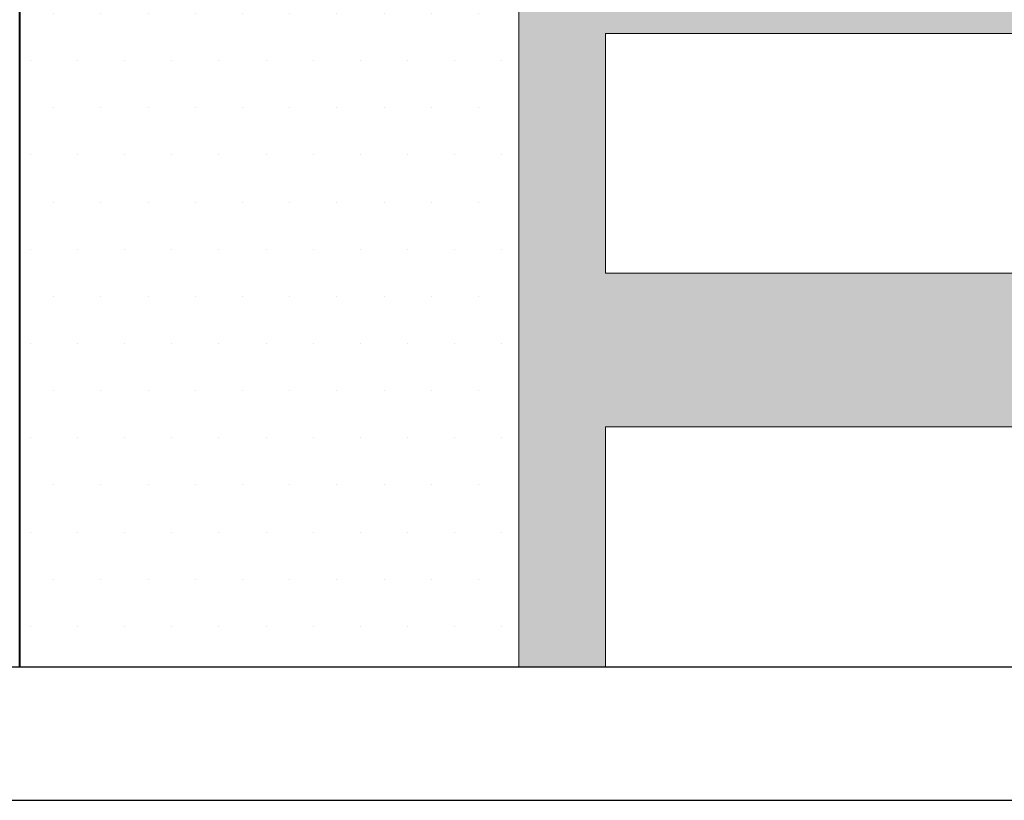
# Model space of a CAD drawing. Units: inches. Extents: x 459864 to 460310, y 324185 to 324787.
# Tile 2 of 112: x 460061 to 460094, y 324195 to 324221. Entities that reach past the tile are written whole.
import ezdxf

# ---------------------------------------------------------------- set-up
doc = ezdxf.new("R2010")
doc.units = ezdxf.units.IN
for name, color, linetype, lineweight in [('A-WALL', 7, 'Continuous', 40), ('C-PROP', 7, 'Continuous', 30), ('L-HRDS', 9, 'Continuous', 18), ('L-SITE-PATT', 252, 'Continuous', 13)]:
    doc.layers.add(name, color=color, linetype=linetype, lineweight=lineweight)

msp = doc.modelspace()

# ---------------------------------------------------------------- hatches: boundary and pattern name
at = {"layer": 'L-SITE-PATT'}
h = msp.add_hatch(dxfattribs=at)
h.set_pattern_fill('DOTS', color=256)
h.paths.add_polyline_path([(460269.804, 324283.483), (460247.115, 324283.483), (460121.929, 324283.483), (460121.929, 324252.473), (460117.429, 324252.473), (460110.124, 324252.473), (460110.124, 324243.287), (460080.83, 324243.287), (460080.83, 324252.473), (460061.115, 324252.473), (460061.115, 324251.882), (460077.909, 324251.882), (460077.909, 324199.483), (460080.83, 324199.483), (460080.83, 324207.553), (460110.124, 324207.553), (460110.124, 324199.483), (460110.813, 324199.483), (460262.115, 324199.483), (460269.804, 324199.483)], flags=17)
edge = h.paths.add_edge_path(flags=0)
edge.add_ellipse((460222.59, 324263.813), major_axis=(-8.485, 8.485), ratio=1, start_angle=405, end_angle=495, ccw=False)
edge.add_line((460214.821, 324254.66), (460214.832, 324254.666))
edge.add_ellipse((460222.59, 324263.813), major_axis=(-8.485, 8.485), ratio=1, start_angle=405, end_angle=495, ccw=False)
edge.add_line((460210.759, 324261.781), (460210.768, 324261.787))
edge.add_ellipse((460222.59, 324263.813), major_axis=(-8.485, 8.485), ratio=1, start_angle=405, end_angle=495, ccw=False)
edge.add_ellipse((460222.59, 324263.813), major_axis=(-8.485, 8.485), ratio=1, start_angle=392.754, end_angle=405, ccw=False)
edge.add_ellipse((460222.59, 324263.813), major_axis=(-8.485, 8.485), ratio=1, start_angle=380.9347, end_angle=392.754, ccw=False)
edge.add_line((460211.337, 324267.985), (460211.34, 324267.985))
edge.add_ellipse((460222.59, 324263.813), major_axis=(-8.485, 8.485), ratio=1, start_angle=380.9347, end_angle=392.754, ccw=False)
edge.add_ellipse((460222.59, 324263.813), major_axis=(-8.485, 8.485), ratio=1, start_angle=347.9015, end_angle=380.9347, ccw=False)
edge.add_ellipse((460222.59, 324263.813), major_axis=(-8.485, 8.485), ratio=1, start_angle=327.0619, end_angle=347.9015, ccw=False)
edge.add_ellipse((460222.59, 324263.813), major_axis=(-8.485, 8.485), ratio=1, start_angle=278.3246, end_angle=327.0619, ccw=False)
edge.add_line((460225.158, 324275.536), (460225.158, 324275.535))
edge.add_ellipse((460222.59, 324263.813), major_axis=(-8.485, 8.485), ratio=1, start_angle=278.3246, end_angle=327.0619, ccw=False)
edge.add_ellipse((460222.59, 324263.813), major_axis=(-8.485, 8.485), ratio=1, start_angle=260.6436, end_angle=278.3246, ccw=False)
edge.add_ellipse((460222.59, 324263.813), major_axis=(-8.485, 8.485), ratio=1, start_angle=225, end_angle=260.6436, ccw=False)
edge.add_line((460234.509, 324265.243), (460234.501, 324265.239))
edge.add_ellipse((460222.59, 324263.813), major_axis=(-8.485, 8.485), ratio=1, start_angle=225, end_angle=260.6436, ccw=False)
edge.add_ellipse((460222.59, 324263.813), major_axis=(-8.485, 8.485), ratio=1, start_angle=495, end_angle=585, ccw=False)
edge.add_line((460234.437, 324261.861), (460234.424, 324261.858))
edge.add_ellipse((460222.59, 324263.813), major_axis=(-8.485, 8.485), ratio=1, start_angle=495, end_angle=585, ccw=False)
edge.add_line((460227.95, 324253.067), (460227.946, 324253.083))
edge.add_ellipse((460222.59, 324263.813), major_axis=(-8.485, 8.485), ratio=1, start_angle=495, end_angle=585, ccw=False)
edge.add_line((460226.223, 324252.369), (460226.211, 324252.38))
edge.add_ellipse((460222.59, 324263.813), major_axis=(-8.485, 8.485), ratio=1, start_angle=495, end_angle=585, ccw=False)
h.paths.add_polyline_path([(460219.651, 324254.347), (460218.461, 324253.545), (460218.275, 324254.789), (460219.642, 324256.542), (460219.625, 324260.848), (460216.11, 324257.333), (460214.35, 324256.978), (460215.416, 324259.356), (460212.524, 324258.496), (460213.137, 324259.93), (460218.507, 324263.813), (460222.59, 324263.813), (460222.59, 324267.807), (460218.176, 324272.212), (460219.026, 324274.639), (460222.59, 324272.811), (460222.59, 324275.423), (460223.057, 324274.825), (460222.675, 324273.492), (460225.912, 324267.135), (460219.625, 324260.848)], flags=0)
edge = h.paths.add_edge_path(flags=0)
edge.add_ellipse((460194.576, 324264.046), major_axis=(-8.485, 8.485), ratio=1, start_angle=495, end_angle=585, ccw=False)
edge.add_line((460199.936, 324253.3), (460199.932, 324253.316))
edge.add_ellipse((460194.576, 324264.046), major_axis=(-8.485, 8.485), ratio=1, start_angle=495, end_angle=585, ccw=False)
edge.add_line((460198.208, 324252.603), (460198.196, 324252.613))
edge.add_ellipse((460194.576, 324264.046), major_axis=(-8.485, 8.485), ratio=1, start_angle=495, end_angle=585, ccw=False)
edge.add_ellipse((460194.576, 324264.046), major_axis=(-8.485, 8.485), ratio=1, start_angle=405, end_angle=495, ccw=False)
edge.add_line((460186.806, 324254.893), (460186.817, 324254.899))
edge.add_ellipse((460194.576, 324264.046), major_axis=(-8.485, 8.485), ratio=1, start_angle=405, end_angle=495, ccw=False)
edge.add_line((460182.744, 324262.014), (460182.753, 324262.02))
edge.add_ellipse((460194.576, 324264.046), major_axis=(-8.485, 8.485), ratio=1, start_angle=405, end_angle=495, ccw=False)
edge.add_ellipse((460194.576, 324264.046), major_axis=(-8.485, 8.485), ratio=1, start_angle=392.754, end_angle=405, ccw=False)
edge.add_ellipse((460194.576, 324264.046), major_axis=(-8.485, 8.485), ratio=1, start_angle=380.9347, end_angle=392.754, ccw=False)
edge.add_line((460183.323, 324268.218), (460183.326, 324268.218))
edge.add_ellipse((460194.576, 324264.046), major_axis=(-8.485, 8.485), ratio=1, start_angle=380.9347, end_angle=392.754, ccw=False)
edge.add_ellipse((460194.576, 324264.046), major_axis=(-8.485, 8.485), ratio=1, start_angle=347.9015, end_angle=380.9347, ccw=False)
edge.add_ellipse((460194.576, 324264.046), major_axis=(-8.485, 8.485), ratio=1, start_angle=327.0619, end_angle=347.9015, ccw=False)
edge.add_ellipse((460194.576, 324264.046), major_axis=(-8.485, 8.485), ratio=1, start_angle=278.3246, end_angle=327.0619, ccw=False)
edge.add_line((460197.144, 324275.769), (460197.143, 324275.768))
edge.add_ellipse((460194.576, 324264.046), major_axis=(-8.485, 8.485), ratio=1, start_angle=278.3246, end_angle=327.0619, ccw=False)
edge.add_ellipse((460194.576, 324264.046), major_axis=(-8.485, 8.485), ratio=1, start_angle=260.6436, end_angle=278.3246, ccw=False)
edge.add_ellipse((460194.576, 324264.046), major_axis=(-8.485, 8.485), ratio=1, start_angle=225, end_angle=260.6436, ccw=False)
edge.add_line((460206.494, 324265.476), (460206.487, 324265.473))
edge.add_ellipse((460194.576, 324264.046), major_axis=(-8.485, 8.485), ratio=1, start_angle=225, end_angle=260.6436, ccw=False)
edge.add_ellipse((460194.576, 324264.046), major_axis=(-8.485, 8.485), ratio=1, start_angle=495, end_angle=585, ccw=False)
edge.add_line((460206.422, 324262.094), (460206.409, 324262.091))
h.paths.add_polyline_path([(460191.61, 324261.081), (460191.637, 324254.58), (460190.447, 324253.778), (460190.261, 324255.023), (460191.628, 324256.775), (460191.61, 324261.081), (460188.096, 324257.566), (460186.335, 324257.211), (460187.402, 324259.589), (460184.509, 324258.729), (460185.123, 324260.163), (460190.493, 324264.046), (460194.576, 324264.046), (460194.576, 324268.04), (460190.161, 324272.446), (460191.011, 324274.872), (460194.576, 324273.044), (460194.576, 324275.657), (460195.043, 324275.058), (460194.661, 324273.725), (460197.897, 324267.368)], flags=0)
edge = h.paths.add_edge_path(flags=0)
edge.add_ellipse((460252.912, 324263.578), major_axis=(-8.485, 8.485), ratio=1, start_angle=405, end_angle=495, ccw=False)
edge.add_line((460241.081, 324261.545), (460241.089, 324261.551))
edge.add_ellipse((460252.912, 324263.578), major_axis=(-8.485, 8.485), ratio=1, start_angle=405, end_angle=495, ccw=False)
edge.add_ellipse((460252.912, 324263.578), major_axis=(-8.485, 8.485), ratio=1, start_angle=392.754, end_angle=405, ccw=False)
edge.add_ellipse((460252.912, 324263.578), major_axis=(-8.485, 8.485), ratio=1, start_angle=380.9347, end_angle=392.754, ccw=False)
edge.add_line((460241.659, 324267.749), (460241.662, 324267.749))
edge.add_ellipse((460252.912, 324263.578), major_axis=(-8.485, 8.485), ratio=1, start_angle=380.9347, end_angle=392.754, ccw=False)
edge.add_ellipse((460252.912, 324263.578), major_axis=(-8.485, 8.485), ratio=1, start_angle=347.9015, end_angle=380.9347, ccw=False)
edge.add_ellipse((460252.912, 324263.578), major_axis=(-8.485, 8.485), ratio=1, start_angle=327.0619, end_angle=347.9015, ccw=False)
edge.add_ellipse((460252.912, 324263.578), major_axis=(-8.485, 8.485), ratio=1, start_angle=278.3246, end_angle=327.0619, ccw=False)
edge.add_line((460255.48, 324275.3), (460255.479, 324275.299))
edge.add_ellipse((460252.912, 324263.578), major_axis=(-8.485, 8.485), ratio=1, start_angle=278.3246, end_angle=327.0619, ccw=False)
edge.add_ellipse((460252.912, 324263.578), major_axis=(-8.485, 8.485), ratio=1, start_angle=260.6436, end_angle=278.3246, ccw=False)
edge.add_ellipse((460252.912, 324263.578), major_axis=(-8.485, 8.485), ratio=1, start_angle=225, end_angle=260.6436, ccw=False)
edge.add_line((460264.83, 324265.007), (460264.823, 324265.004))
edge.add_ellipse((460252.912, 324263.578), major_axis=(-8.485, 8.485), ratio=1, start_angle=225, end_angle=260.6436, ccw=False)
edge.add_ellipse((460252.912, 324263.578), major_axis=(-8.485, 8.485), ratio=1, start_angle=495, end_angle=585, ccw=False)
edge.add_line((460264.758, 324261.626), (460264.745, 324261.622))
edge.add_ellipse((460252.912, 324263.578), major_axis=(-8.485, 8.485), ratio=1, start_angle=495, end_angle=585, ccw=False)
edge.add_line((460258.272, 324252.832), (460258.268, 324252.848))
edge.add_ellipse((460252.912, 324263.578), major_axis=(-8.485, 8.485), ratio=1, start_angle=495, end_angle=585, ccw=False)
edge.add_line((460256.545, 324252.134), (460256.533, 324252.144))
edge.add_ellipse((460252.912, 324263.578), major_axis=(-8.485, 8.485), ratio=1, start_angle=495, end_angle=585, ccw=False)
edge.add_ellipse((460252.912, 324263.578), major_axis=(-8.485, 8.485), ratio=1, start_angle=405, end_angle=495, ccw=False)
edge.add_line((460245.143, 324254.424), (460245.153, 324254.43))
h.paths.add_polyline_path([(460244.672, 324256.742), (460245.738, 324259.12), (460242.846, 324258.26), (460243.459, 324259.694), (460248.829, 324263.578), (460252.912, 324263.578), (460252.912, 324267.571), (460248.497, 324271.977), (460249.348, 324274.403), (460252.912, 324272.576), (460252.912, 324275.188), (460253.379, 324274.589), (460252.997, 324273.257), (460256.233, 324266.899), (460249.946, 324260.612), (460249.973, 324254.111), (460248.783, 324253.309), (460248.597, 324254.554), (460249.964, 324256.306), (460249.946, 324260.612), (460246.432, 324257.097)], flags=0)
edge = h.paths.add_edge_path(flags=0)
edge.add_ellipse((460167.439, 324262.833), major_axis=(-8.485, 8.485), ratio=1, start_angle=495, end_angle=585, ccw=False)
edge.add_line((460172.799, 324252.087), (460172.795, 324252.103))
edge.add_ellipse((460167.439, 324262.833), major_axis=(-8.485, 8.485), ratio=1, start_angle=495, end_angle=585, ccw=False)
edge.add_line((460171.071, 324251.389), (460171.059, 324251.399))
edge.add_ellipse((460167.439, 324262.833), major_axis=(-8.485, 8.485), ratio=1, start_angle=495, end_angle=585, ccw=False)
edge.add_ellipse((460167.439, 324262.833), major_axis=(-8.485, 8.485), ratio=1, start_angle=405, end_angle=495, ccw=False)
edge.add_line((460159.669, 324253.679), (460159.68, 324253.685))
edge.add_ellipse((460167.439, 324262.833), major_axis=(-8.485, 8.485), ratio=1, start_angle=405, end_angle=495, ccw=False)
edge.add_line((460155.607, 324260.8), (460155.616, 324260.806))
edge.add_ellipse((460167.439, 324262.833), major_axis=(-8.485, 8.485), ratio=1, start_angle=405, end_angle=495, ccw=False)
edge.add_ellipse((460167.439, 324262.833), major_axis=(-8.485, 8.485), ratio=1, start_angle=392.754, end_angle=405, ccw=False)
edge.add_ellipse((460167.439, 324262.833), major_axis=(-8.485, 8.485), ratio=1, start_angle=380.9347, end_angle=392.754, ccw=False)
edge.add_line((460156.185, 324267.005), (460156.189, 324267.005))
edge.add_ellipse((460167.439, 324262.833), major_axis=(-8.485, 8.485), ratio=1, start_angle=380.9347, end_angle=392.754, ccw=False)
edge.add_ellipse((460167.439, 324262.833), major_axis=(-8.485, 8.485), ratio=1, start_angle=347.9015, end_angle=380.9347, ccw=False)
edge.add_ellipse((460167.439, 324262.833), major_axis=(-8.485, 8.485), ratio=1, start_angle=327.0619, end_angle=347.9015, ccw=False)
edge.add_ellipse((460167.439, 324262.833), major_axis=(-8.485, 8.485), ratio=1, start_angle=278.3246, end_angle=327.0619, ccw=False)
edge.add_line((460170.007, 324274.556), (460170.006, 324274.554))
edge.add_ellipse((460167.439, 324262.833), major_axis=(-8.485, 8.485), ratio=1, start_angle=278.3246, end_angle=327.0619, ccw=False)
edge.add_ellipse((460167.439, 324262.833), major_axis=(-8.485, 8.485), ratio=1, start_angle=260.6436, end_angle=278.3246, ccw=False)
edge.add_ellipse((460167.439, 324262.833), major_axis=(-8.485, 8.485), ratio=1, start_angle=225, end_angle=260.6436, ccw=False)
edge.add_line((460179.357, 324264.262), (460179.35, 324264.259))
edge.add_ellipse((460167.439, 324262.833), major_axis=(-8.485, 8.485), ratio=1, start_angle=225, end_angle=260.6436, ccw=False)
edge.add_ellipse((460167.439, 324262.833), major_axis=(-8.485, 8.485), ratio=1, start_angle=495, end_angle=585, ccw=False)
edge.add_line((460179.285, 324260.881), (460179.272, 324260.877))
h.paths.add_polyline_path([(460164.473, 324259.867), (460164.5, 324253.366), (460163.31, 324252.565), (460163.124, 324253.809), (460164.491, 324255.561), (460164.473, 324259.867), (460160.958, 324256.353), (460159.198, 324255.998), (460160.265, 324258.375), (460157.372, 324257.515), (460157.986, 324258.949), (460163.356, 324262.833), (460167.439, 324262.833), (460167.439, 324266.826), (460163.024, 324271.232), (460163.874, 324273.659), (460167.439, 324271.831), (460167.439, 324274.443), (460167.905, 324273.844), (460167.524, 324272.512), (460170.76, 324266.154)], flags=0)
edge = h.paths.add_edge_path(flags=0)
edge.add_ellipse((460140.758, 324262.37), major_axis=(-8.485, 8.485), ratio=1, start_angle=495, end_angle=585, ccw=False)
edge.add_line((460146.118, 324251.624), (460146.114, 324251.639))
edge.add_ellipse((460140.758, 324262.37), major_axis=(-8.485, 8.485), ratio=1, start_angle=495, end_angle=585, ccw=False)
edge.add_line((460144.391, 324250.926), (460144.379, 324250.936))
edge.add_ellipse((460140.758, 324262.37), major_axis=(-8.485, 8.485), ratio=1, start_angle=495, end_angle=585, ccw=False)
edge.add_ellipse((460140.758, 324262.37), major_axis=(-8.485, 8.485), ratio=1, start_angle=405, end_angle=495, ccw=False)
edge.add_line((460132.989, 324253.216), (460132.999, 324253.222))
edge.add_ellipse((460140.758, 324262.37), major_axis=(-8.485, 8.485), ratio=1, start_angle=405, end_angle=495, ccw=False)
edge.add_line((460128.927, 324260.337), (460128.935, 324260.343))
edge.add_ellipse((460140.758, 324262.37), major_axis=(-8.485, 8.485), ratio=1, start_angle=405, end_angle=495, ccw=False)
edge.add_ellipse((460140.758, 324262.37), major_axis=(-8.485, 8.485), ratio=1, start_angle=392.754, end_angle=405, ccw=False)
edge.add_ellipse((460140.758, 324262.37), major_axis=(-8.485, 8.485), ratio=1, start_angle=380.9347, end_angle=392.754, ccw=False)
edge.add_line((460129.505, 324266.541), (460129.508, 324266.541))
edge.add_ellipse((460140.758, 324262.37), major_axis=(-8.485, 8.485), ratio=1, start_angle=380.9347, end_angle=392.754, ccw=False)
edge.add_ellipse((460140.758, 324262.37), major_axis=(-8.485, 8.485), ratio=1, start_angle=347.9015, end_angle=380.9347, ccw=False)
edge.add_ellipse((460140.758, 324262.37), major_axis=(-8.485, 8.485), ratio=1, start_angle=327.0619, end_angle=347.9015, ccw=False)
edge.add_ellipse((460140.758, 324262.37), major_axis=(-8.485, 8.485), ratio=1, start_angle=278.3246, end_angle=327.0619, ccw=False)
edge.add_line((460143.326, 324274.092), (460143.325, 324274.091))
edge.add_ellipse((460140.758, 324262.37), major_axis=(-8.485, 8.485), ratio=1, start_angle=278.3246, end_angle=327.0619, ccw=False)
edge.add_ellipse((460140.758, 324262.37), major_axis=(-8.485, 8.485), ratio=1, start_angle=260.6436, end_angle=278.3246, ccw=False)
edge.add_ellipse((460140.758, 324262.37), major_axis=(-8.485, 8.485), ratio=1, start_angle=225, end_angle=260.6436, ccw=False)
edge.add_line((460152.677, 324263.799), (460152.669, 324263.796))
edge.add_ellipse((460140.758, 324262.37), major_axis=(-8.485, 8.485), ratio=1, start_angle=225, end_angle=260.6436, ccw=False)
edge.add_ellipse((460140.758, 324262.37), major_axis=(-8.485, 8.485), ratio=1, start_angle=495, end_angle=585, ccw=False)
edge.add_line((460152.604, 324260.418), (460152.592, 324260.414))
h.paths.add_polyline_path([(460137.792, 324259.404), (460137.819, 324252.903), (460136.629, 324252.101), (460136.443, 324253.346), (460137.81, 324255.098), (460137.792, 324259.404), (460134.278, 324255.889), (460132.518, 324255.534), (460133.584, 324257.912), (460130.692, 324257.052), (460131.305, 324258.486), (460136.675, 324262.37), (460140.758, 324262.37), (460140.758, 324266.363), (460136.343, 324270.769), (460137.194, 324273.195), (460140.758, 324271.367), (460140.758, 324273.98), (460141.225, 324273.381), (460140.843, 324272.049), (460144.079, 324265.691)], flags=0)
h.paths.add_polyline_path([(460110.124, 324227.414), (460080.83, 324227.414), (460080.83, 324235.484), (460110.124, 324235.484)], flags=16)
h.paths.add_polyline_path([(460110.124, 324220.797), (460110.124, 324212.727), (460080.83, 324212.727), (460080.83, 324220.797)], flags=16)
h.paths.add_polyline_path([(460269.804, 324283.483), (460247.115, 324283.483), (460121.929, 324283.483), (460121.929, 324252.473), (460117.429, 324252.473), (460110.124, 324252.473), (460110.124, 324243.287), (460080.83, 324243.287), (460080.83, 324252.473), (460061.115, 324252.473), (460061.115, 324251.882), (460077.909, 324251.882), (460077.909, 324199.483), (460080.83, 324199.483), (460080.83, 324207.553), (460110.124, 324207.553), (460110.124, 324199.483), (460262.115, 324199.483), (460269.804, 324199.483)], flags=17)
h.paths.add_polyline_path([(460219.651, 324254.347), (460218.461, 324253.545), (460218.275, 324254.789), (460219.642, 324256.542), (460219.625, 324260.848), (460216.11, 324257.333), (460214.35, 324256.978), (460215.416, 324259.356), (460212.524, 324258.496), (460213.137, 324259.93), (460218.507, 324263.813), (460222.59, 324263.813), (460220.18, 324266.223), (460215.461, 324265.308), (460211.835, 324266.137), (460216.247, 324267.985), (460218.418, 324267.985), (460222.59, 324263.813), (460222.59, 324267.807), (460218.176, 324272.212), (460219.026, 324274.639), (460222.59, 324272.811), (460222.59, 324275.423), (460223.057, 324274.825), (460222.675, 324273.492), (460225.912, 324267.135), (460222.59, 324263.813), (460231.383, 324263.813), (460228.485, 324262.488), (460224.425, 324261.978), (460228.68, 324257.724), (460228.966, 324254.791), (460227.142, 324256.537), (460227.542, 324254.819), (460227.333, 324253.614), (460222.59, 324259.985), (460222.59, 324255.497), (460221.377, 324256.541), (460220.576, 324261.799), (460219.625, 324260.848)], flags=0)
h.paths.add_polyline_path([(460199.127, 324256.77), (460199.528, 324255.052), (460199.319, 324253.848), (460194.576, 324260.218), (460194.576, 324255.73), (460193.363, 324256.774), (460192.561, 324262.032), (460191.61, 324261.081), (460191.637, 324254.58), (460190.447, 324253.778), (460190.261, 324255.023), (460191.628, 324256.775), (460191.61, 324261.081), (460188.096, 324257.566), (460186.335, 324257.211), (460187.402, 324259.589), (460184.509, 324258.729), (460185.123, 324260.163), (460190.493, 324264.046), (460194.576, 324264.046), (460192.166, 324266.456), (460187.446, 324265.541), (460183.82, 324266.37), (460188.232, 324268.218), (460190.404, 324268.218), (460194.576, 324264.046), (460194.576, 324268.04), (460190.161, 324272.446), (460191.011, 324274.872), (460194.576, 324273.044), (460194.576, 324275.657), (460195.043, 324275.058), (460194.661, 324273.725), (460197.897, 324267.368), (460194.576, 324264.046), (460203.368, 324264.046), (460200.47, 324262.721), (460196.411, 324262.212), (460200.665, 324257.957), (460200.951, 324255.024)], flags=0)
h.paths.add_polyline_path([(460244.672, 324256.742), (460245.738, 324259.12), (460242.846, 324258.26), (460243.459, 324259.694), (460248.829, 324263.578), (460252.912, 324263.578), (460250.502, 324265.987), (460245.783, 324265.072), (460242.156, 324265.901), (460246.568, 324267.749), (460248.74, 324267.749), (460252.912, 324263.578), (460252.912, 324267.571), (460248.497, 324271.977), (460249.348, 324274.403), (460252.912, 324272.576), (460252.912, 324275.188), (460253.379, 324274.589), (460252.997, 324273.257), (460256.233, 324266.899), (460252.912, 324263.578), (460261.705, 324263.578), (460258.806, 324262.252), (460254.747, 324261.743), (460259.002, 324257.488), (460259.288, 324254.555), (460257.463, 324256.301), (460257.864, 324254.583), (460257.655, 324253.379), (460252.912, 324259.749), (460252.912, 324255.261), (460251.699, 324256.305), (460250.897, 324261.563), (460249.946, 324260.612), (460249.973, 324254.111), (460248.783, 324253.309), (460248.597, 324254.554), (460249.964, 324256.306), (460249.946, 324260.612), (460246.432, 324257.097)], flags=0)
h.paths.add_polyline_path([(460173.528, 324256.743), (460173.814, 324253.811), (460171.99, 324255.556), (460172.39, 324253.838), (460172.182, 324252.634), (460167.439, 324259.004), (460167.439, 324254.516), (460166.226, 324255.56), (460165.424, 324260.818), (460164.473, 324259.867), (460164.5, 324253.366), (460163.31, 324252.565), (460163.124, 324253.809), (460164.491, 324255.561), (460164.473, 324259.867), (460160.958, 324256.353), (460159.198, 324255.998), (460160.265, 324258.375), (460157.372, 324257.515), (460157.986, 324258.949), (460163.356, 324262.833), (460167.439, 324262.833), (460165.029, 324265.243), (460160.309, 324264.327), (460156.683, 324265.156), (460161.095, 324267.005), (460163.267, 324267.005), (460167.439, 324262.833), (460167.439, 324266.826), (460163.024, 324271.232), (460163.874, 324273.659), (460167.439, 324271.831), (460167.439, 324274.443), (460167.905, 324273.844), (460167.524, 324272.512), (460170.76, 324266.154), (460167.439, 324262.833), (460176.231, 324262.833), (460173.333, 324261.507), (460169.274, 324260.998)], flags=0)
h.paths.add_polyline_path([(460146.848, 324256.28), (460147.134, 324253.347), (460145.31, 324255.093), (460145.71, 324253.375), (460145.501, 324252.171), (460140.758, 324258.541), (460140.758, 324254.053), (460139.545, 324255.097), (460138.744, 324260.355), (460137.792, 324259.404), (460137.819, 324252.903), (460136.629, 324252.101), (460136.443, 324253.346), (460137.81, 324255.098), (460137.792, 324259.404), (460134.278, 324255.889), (460132.518, 324255.534), (460133.584, 324257.912), (460130.692, 324257.052), (460131.305, 324258.486), (460136.675, 324262.37), (460140.758, 324262.37), (460138.348, 324264.779), (460133.629, 324263.864), (460130.002, 324264.693), (460134.414, 324266.541), (460136.586, 324266.541), (460140.758, 324262.37), (460140.758, 324266.363), (460136.343, 324270.769), (460137.194, 324273.195), (460140.758, 324271.367), (460140.758, 324273.98), (460141.225, 324273.381), (460140.843, 324272.049), (460144.079, 324265.691), (460140.758, 324262.37), (460149.551, 324262.37), (460146.653, 324261.044), (460142.593, 324260.535)], flags=0)
edge = h.paths.add_edge_path()
edge.add_line((460269.804, 324272.549), (460260.881, 324272.549))
edge.add_ellipse((460252.912, 324263.578), major_axis=(-8.485, 8.485), ratio=1, start_angle=260.6436, end_angle=273.3846, ccw=False)
edge.add_line((460262.283, 324271.092), (460262.261, 324271.091))
edge.add_ellipse((460252.912, 324263.578), major_axis=(-8.485, 8.485), ratio=1, start_angle=260.6436, end_angle=273.3846, ccw=False)
edge.add_ellipse((460252.912, 324263.578), major_axis=(-8.485, 8.485), ratio=1, start_angle=225, end_angle=260.6436, ccw=False)
edge.add_line((460263.609, 324269.063), (460263.572, 324269.058))
edge.add_ellipse((460252.912, 324263.578), major_axis=(-8.485, 8.485), ratio=1, start_angle=225, end_angle=260.6436, ccw=False)
edge.add_line((460264.615, 324266.306), (460264.585, 324266.305))
edge.add_ellipse((460252.912, 324263.578), major_axis=(-8.485, 8.485), ratio=1, start_angle=225, end_angle=260.6436, ccw=False)
edge.add_line((460264.83, 324265.007), (460264.823, 324265.004))
edge.add_ellipse((460252.912, 324263.578), major_axis=(-8.485, 8.485), ratio=1, start_angle=225, end_angle=260.6436, ccw=False)
edge.add_ellipse((460252.912, 324263.578), major_axis=(-8.485, 8.485), ratio=1, start_angle=495, end_angle=585, ccw=False)
edge.add_line((460264.758, 324261.626), (460264.745, 324261.622))
edge.add_ellipse((460252.912, 324263.578), major_axis=(-8.485, 8.485), ratio=1, start_angle=495, end_angle=585, ccw=False)
edge.add_line((460263.442, 324257.739), (460263.389, 324257.779))
edge.add_ellipse((460252.912, 324263.578), major_axis=(-8.485, 8.485), ratio=1, start_angle=495, end_angle=585, ccw=False)
edge.add_line((460258.128, 324252.744), (460258.102, 324252.779))
edge.add_ellipse((460252.912, 324263.578), major_axis=(-8.485, 8.485), ratio=1, start_angle=495, end_angle=585, ccw=False)
edge.add_line((460256.545, 324252.134), (460256.533, 324252.144))
edge.add_ellipse((460252.912, 324263.578), major_axis=(-8.485, 8.485), ratio=1, start_angle=495, end_angle=585, ccw=False)
edge.add_ellipse((460252.912, 324263.578), major_axis=(-8.485, 8.485), ratio=1, start_angle=405, end_angle=495, ccw=False)
edge.add_line((460250.594, 324251.78), (460250.605, 324251.82))
edge.add_ellipse((460252.912, 324263.578), major_axis=(-8.485, 8.485), ratio=1, start_angle=405, end_angle=495, ccw=False)
edge.add_line((460245.143, 324254.424), (460245.153, 324254.43))
edge.add_ellipse((460252.912, 324263.578), major_axis=(-8.485, 8.485), ratio=1, start_angle=405, end_angle=495, ccw=False)
edge.add_line((460243.525, 324256.059), (460243.56, 324256.091))
edge.add_ellipse((460252.912, 324263.578), major_axis=(-8.485, 8.485), ratio=1, start_angle=405, end_angle=495, ccw=False)
edge.add_line((460241.44, 324259.893), (460241.522, 324259.896))
edge.add_ellipse((460252.912, 324263.578), major_axis=(-8.485, 8.485), ratio=1, start_angle=405, end_angle=495, ccw=False)
edge.add_line((460241.081, 324261.545), (460241.089, 324261.551))
edge.add_ellipse((460252.912, 324263.578), major_axis=(-8.485, 8.485), ratio=1, start_angle=405, end_angle=495, ccw=False)
edge.add_ellipse((460252.912, 324263.578), major_axis=(-8.485, 8.485), ratio=1, start_angle=392.754, end_angle=405, ccw=False)
edge.add_line((460241.05, 324265.438), (460241.063, 324265.443))
edge.add_ellipse((460252.912, 324263.578), major_axis=(-8.485, 8.485), ratio=1, start_angle=392.754, end_angle=405, ccw=False)
edge.add_ellipse((460252.912, 324263.578), major_axis=(-8.485, 8.485), ratio=1, start_angle=380.9347, end_angle=392.754, ccw=False)
edge.add_line((460241.452, 324267.176), (460241.469, 324267.171))
edge.add_ellipse((460252.912, 324263.578), major_axis=(-8.485, 8.485), ratio=1, start_angle=380.9347, end_angle=392.754, ccw=False)
edge.add_line((460241.659, 324267.749), (460241.662, 324267.749))
edge.add_ellipse((460252.912, 324263.578), major_axis=(-8.485, 8.485), ratio=1, start_angle=380.9347, end_angle=392.754, ccw=False)
edge.add_ellipse((460252.912, 324263.578), major_axis=(-8.485, 8.485), ratio=1, start_angle=356.6154, end_angle=380.9347, ccw=False)
edge.add_line((460244.88, 324272.488), (460244.713, 324272.549))
edge.add_line((460244.713, 324272.549), (460230.817, 324272.549))
edge.add_ellipse((460222.59, 324263.813), major_axis=(-8.485, 8.485), ratio=1, start_angle=260.6436, end_angle=271.7178, ccw=False)
edge.add_ellipse((460222.59, 324263.813), major_axis=(-8.485, 8.485), ratio=1, start_angle=225, end_angle=260.6436, ccw=False)
edge.add_line((460233.287, 324269.299), (460233.25, 324269.294))
edge.add_ellipse((460222.59, 324263.813), major_axis=(-8.485, 8.485), ratio=1, start_angle=225, end_angle=260.6436, ccw=False)
edge.add_line((460234.294, 324266.541), (460234.264, 324266.541))
edge.add_ellipse((460222.59, 324263.813), major_axis=(-8.485, 8.485), ratio=1, start_angle=225, end_angle=260.6436, ccw=False)
edge.add_line((460234.509, 324265.243), (460234.501, 324265.239))
edge.add_ellipse((460222.59, 324263.813), major_axis=(-8.485, 8.485), ratio=1, start_angle=225, end_angle=260.6436, ccw=False)
edge.add_ellipse((460222.59, 324263.813), major_axis=(-8.485, 8.485), ratio=1, start_angle=495, end_angle=585, ccw=False)
edge.add_line((460234.437, 324261.861), (460234.424, 324261.858))
edge.add_ellipse((460222.59, 324263.813), major_axis=(-8.485, 8.485), ratio=1, start_angle=495, end_angle=585, ccw=False)
edge.add_line((460233.121, 324257.975), (460233.068, 324258.015))
edge.add_ellipse((460222.59, 324263.813), major_axis=(-8.485, 8.485), ratio=1, start_angle=495, end_angle=585, ccw=False)
edge.add_line((460227.806, 324252.979), (460227.78, 324253.014))
edge.add_ellipse((460222.59, 324263.813), major_axis=(-8.485, 8.485), ratio=1, start_angle=495, end_angle=585, ccw=False)
edge.add_line((460226.223, 324252.369), (460226.211, 324252.38))
edge.add_ellipse((460222.59, 324263.813), major_axis=(-8.485, 8.485), ratio=1, start_angle=495, end_angle=585, ccw=False)
edge.add_ellipse((460222.59, 324263.813), major_axis=(-8.485, 8.485), ratio=1, start_angle=405, end_angle=495, ccw=False)
edge.add_line((460220.272, 324252.016), (460220.283, 324252.055))
edge.add_ellipse((460222.59, 324263.813), major_axis=(-8.485, 8.485), ratio=1, start_angle=405, end_angle=495, ccw=False)
edge.add_line((460214.821, 324254.66), (460214.832, 324254.666))
edge.add_ellipse((460222.59, 324263.813), major_axis=(-8.485, 8.485), ratio=1, start_angle=405, end_angle=495, ccw=False)
edge.add_line((460213.203, 324256.295), (460213.239, 324256.327))
edge.add_ellipse((460222.59, 324263.813), major_axis=(-8.485, 8.485), ratio=1, start_angle=405, end_angle=495, ccw=False)
edge.add_line((460211.118, 324260.128), (460211.201, 324260.131))
edge.add_ellipse((460222.59, 324263.813), major_axis=(-8.485, 8.485), ratio=1, start_angle=405, end_angle=495, ccw=False)
edge.add_line((460210.759, 324261.781), (460210.768, 324261.787))
edge.add_ellipse((460222.59, 324263.813), major_axis=(-8.485, 8.485), ratio=1, start_angle=405, end_angle=495, ccw=False)
edge.add_ellipse((460222.59, 324263.813), major_axis=(-8.485, 8.485), ratio=1, start_angle=392.754, end_angle=405, ccw=False)
edge.add_line((460210.729, 324265.673), (460210.741, 324265.678))
edge.add_ellipse((460222.59, 324263.813), major_axis=(-8.485, 8.485), ratio=1, start_angle=392.754, end_angle=405, ccw=False)
edge.add_ellipse((460222.59, 324263.813), major_axis=(-8.485, 8.485), ratio=1, start_angle=380.9347, end_angle=392.754, ccw=False)
edge.add_line((460211.13, 324267.412), (460211.147, 324267.407))
edge.add_ellipse((460222.59, 324263.813), major_axis=(-8.485, 8.485), ratio=1, start_angle=380.9347, end_angle=392.754, ccw=False)
edge.add_line((460211.337, 324267.985), (460211.34, 324267.985))
edge.add_ellipse((460222.59, 324263.813), major_axis=(-8.485, 8.485), ratio=1, start_angle=380.9347, end_angle=392.754, ccw=False)
edge.add_ellipse((460222.59, 324263.813), major_axis=(-8.485, 8.485), ratio=1, start_angle=358.2822, end_angle=380.9347, ccw=False)
edge.add_line((460213.705, 324271.902), (460213.709, 324271.869))
edge.add_ellipse((460222.59, 324263.813), major_axis=(-8.485, 8.485), ratio=1, start_angle=358.2822, end_angle=380.9347, ccw=False)
edge.add_line((460214.363, 324272.549), (460203.078, 324272.549))
edge.add_line((460203.078, 324272.549), (460203.06, 324272.531))
edge.add_ellipse((460194.576, 324264.046), major_axis=(-8.485, 8.485), ratio=1, start_angle=260.6436, end_angle=270.1168, ccw=False)
edge.add_line((460203.957, 324271.561), (460203.921, 324271.56))
edge.add_ellipse((460194.576, 324264.046), major_axis=(-8.485, 8.485), ratio=1, start_angle=260.6436, end_angle=270.1168, ccw=False)
edge.add_ellipse((460194.576, 324264.046), major_axis=(-8.485, 8.485), ratio=1, start_angle=225, end_angle=260.6436, ccw=False)
edge.add_line((460205.272, 324269.532), (460205.235, 324269.527))
edge.add_ellipse((460194.576, 324264.046), major_axis=(-8.485, 8.485), ratio=1, start_angle=225, end_angle=260.6436, ccw=False)
edge.add_line((460206.279, 324266.774), (460206.249, 324266.774))
edge.add_ellipse((460194.576, 324264.046), major_axis=(-8.485, 8.485), ratio=1, start_angle=225, end_angle=260.6436, ccw=False)
edge.add_line((460206.494, 324265.476), (460206.487, 324265.473))
edge.add_ellipse((460194.576, 324264.046), major_axis=(-8.485, 8.485), ratio=1, start_angle=225, end_angle=260.6436, ccw=False)
edge.add_ellipse((460194.576, 324264.046), major_axis=(-8.485, 8.485), ratio=1, start_angle=495, end_angle=585, ccw=False)
edge.add_line((460206.422, 324262.094), (460206.409, 324262.091))
edge.add_ellipse((460194.576, 324264.046), major_axis=(-8.485, 8.485), ratio=1, start_angle=495, end_angle=585, ccw=False)
edge.add_line((460205.106, 324258.208), (460205.053, 324258.248))
edge.add_ellipse((460194.576, 324264.046), major_axis=(-8.485, 8.485), ratio=1, start_angle=495, end_angle=585, ccw=False)
edge.add_line((460199.792, 324253.212), (460199.766, 324253.248))
edge.add_ellipse((460194.576, 324264.046), major_axis=(-8.485, 8.485), ratio=1, start_angle=495, end_angle=585, ccw=False)
edge.add_line((460198.208, 324252.603), (460198.196, 324252.613))
edge.add_ellipse((460194.576, 324264.046), major_axis=(-8.485, 8.485), ratio=1, start_angle=495, end_angle=585, ccw=False)
edge.add_ellipse((460194.576, 324264.046), major_axis=(-8.485, 8.485), ratio=1, start_angle=405, end_angle=495, ccw=False)
edge.add_line((460192.258, 324252.249), (460192.268, 324252.289))
edge.add_ellipse((460194.576, 324264.046), major_axis=(-8.485, 8.485), ratio=1, start_angle=405, end_angle=495, ccw=False)
edge.add_line((460186.806, 324254.893), (460186.817, 324254.899))
edge.add_ellipse((460194.576, 324264.046), major_axis=(-8.485, 8.485), ratio=1, start_angle=405, end_angle=495, ccw=False)
edge.add_line((460185.188, 324256.528), (460185.224, 324256.56))
edge.add_ellipse((460194.576, 324264.046), major_axis=(-8.485, 8.485), ratio=1, start_angle=405, end_angle=495, ccw=False)
edge.add_line((460183.104, 324260.362), (460183.186, 324260.365))
edge.add_ellipse((460194.576, 324264.046), major_axis=(-8.485, 8.485), ratio=1, start_angle=405, end_angle=495, ccw=False)
edge.add_line((460182.744, 324262.014), (460182.753, 324262.02))
edge.add_ellipse((460194.576, 324264.046), major_axis=(-8.485, 8.485), ratio=1, start_angle=405, end_angle=495, ccw=False)
edge.add_ellipse((460194.576, 324264.046), major_axis=(-8.485, 8.485), ratio=1, start_angle=392.754, end_angle=405, ccw=False)
edge.add_line((460182.714, 324265.906), (460182.726, 324265.912))
edge.add_ellipse((460194.576, 324264.046), major_axis=(-8.485, 8.485), ratio=1, start_angle=392.754, end_angle=405, ccw=False)
edge.add_ellipse((460194.576, 324264.046), major_axis=(-8.485, 8.485), ratio=1, start_angle=380.9347, end_angle=392.754, ccw=False)
edge.add_line((460183.116, 324267.645), (460183.133, 324267.64))
edge.add_ellipse((460194.576, 324264.046), major_axis=(-8.485, 8.485), ratio=1, start_angle=380.9347, end_angle=392.754, ccw=False)
edge.add_line((460183.323, 324268.218), (460183.326, 324268.218))
edge.add_ellipse((460194.576, 324264.046), major_axis=(-8.485, 8.485), ratio=1, start_angle=380.9347, end_angle=392.754, ccw=False)
edge.add_ellipse((460194.576, 324264.046), major_axis=(-8.485, 8.485), ratio=1, start_angle=359.8832, end_angle=380.9347, ccw=False)
edge.add_line((460184.491, 324270.611), (460184.553, 324270.611))
edge.add_ellipse((460194.576, 324264.046), major_axis=(-8.485, 8.485), ratio=1, start_angle=359.8832, end_angle=380.9347, ccw=False)
edge.add_line((460185.346, 324271.76), (460185.379, 324271.728))
edge.add_ellipse((460194.576, 324264.046), major_axis=(-8.485, 8.485), ratio=1, start_angle=359.8832, end_angle=380.9347, ccw=False)
edge.add_line((460185.697, 324272.086), (460185.633, 324272.549))
edge.add_line((460185.633, 324272.549), (460174.683, 324272.549))
edge.add_line((460174.683, 324272.549), (460174.606, 324272.457))
edge.add_ellipse((460167.439, 324262.833), major_axis=(-8.485, 8.485), ratio=1, start_angle=260.6436, end_angle=278.3246, ccw=False)
edge.add_ellipse((460167.439, 324262.833), major_axis=(-8.485, 8.485), ratio=1, start_angle=225, end_angle=260.6436, ccw=False)
edge.add_line((460178.135, 324268.318), (460178.098, 324268.313))
edge.add_ellipse((460167.439, 324262.833), major_axis=(-8.485, 8.485), ratio=1, start_angle=225, end_angle=260.6436, ccw=False)
edge.add_line((460179.142, 324265.561), (460179.112, 324265.56))
edge.add_ellipse((460167.439, 324262.833), major_axis=(-8.485, 8.485), ratio=1, start_angle=225, end_angle=260.6436, ccw=False)
edge.add_line((460179.357, 324264.262), (460179.35, 324264.259))
edge.add_ellipse((460167.439, 324262.833), major_axis=(-8.485, 8.485), ratio=1, start_angle=225, end_angle=260.6436, ccw=False)
edge.add_ellipse((460167.439, 324262.833), major_axis=(-8.485, 8.485), ratio=1, start_angle=495, end_angle=585, ccw=False)
edge.add_line((460179.285, 324260.881), (460179.272, 324260.877))
edge.add_ellipse((460167.439, 324262.833), major_axis=(-8.485, 8.485), ratio=1, start_angle=495, end_angle=585, ccw=False)
edge.add_line((460177.969, 324256.994), (460177.916, 324257.034))
edge.add_ellipse((460167.439, 324262.833), major_axis=(-8.485, 8.485), ratio=1, start_angle=495, end_angle=585, ccw=False)
edge.add_line((460172.655, 324251.999), (460172.629, 324252.034))
edge.add_ellipse((460167.439, 324262.833), major_axis=(-8.485, 8.485), ratio=1, start_angle=495, end_angle=585, ccw=False)
edge.add_line((460171.071, 324251.389), (460171.059, 324251.399))
edge.add_ellipse((460167.439, 324262.833), major_axis=(-8.485, 8.485), ratio=1, start_angle=495, end_angle=585, ccw=False)
edge.add_ellipse((460167.439, 324262.833), major_axis=(-8.485, 8.485), ratio=1, start_angle=405, end_angle=495, ccw=False)
edge.add_line((460165.121, 324251.036), (460165.131, 324251.075))
edge.add_ellipse((460167.439, 324262.833), major_axis=(-8.485, 8.485), ratio=1, start_angle=405, end_angle=495, ccw=False)
edge.add_line((460159.669, 324253.679), (460159.68, 324253.685))
edge.add_ellipse((460167.439, 324262.833), major_axis=(-8.485, 8.485), ratio=1, start_angle=405, end_angle=495, ccw=False)
edge.add_line((460158.051, 324255.314), (460158.087, 324255.347))
edge.add_ellipse((460167.439, 324262.833), major_axis=(-8.485, 8.485), ratio=1, start_angle=405, end_angle=495, ccw=False)
edge.add_line((460155.967, 324259.148), (460156.049, 324259.151))
edge.add_ellipse((460167.439, 324262.833), major_axis=(-8.485, 8.485), ratio=1, start_angle=405, end_angle=495, ccw=False)
edge.add_line((460155.607, 324260.8), (460155.616, 324260.806))
edge.add_ellipse((460167.439, 324262.833), major_axis=(-8.485, 8.485), ratio=1, start_angle=405, end_angle=495, ccw=False)
edge.add_ellipse((460167.439, 324262.833), major_axis=(-8.485, 8.485), ratio=1, start_angle=392.754, end_angle=405, ccw=False)
edge.add_line((460155.577, 324264.693), (460155.589, 324264.698))
edge.add_ellipse((460167.439, 324262.833), major_axis=(-8.485, 8.485), ratio=1, start_angle=392.754, end_angle=405, ccw=False)
edge.add_ellipse((460167.439, 324262.833), major_axis=(-8.485, 8.485), ratio=1, start_angle=380.9347, end_angle=392.754, ccw=False)
edge.add_line((460155.979, 324266.432), (460155.996, 324266.426))
edge.add_ellipse((460167.439, 324262.833), major_axis=(-8.485, 8.485), ratio=1, start_angle=380.9347, end_angle=392.754, ccw=False)
edge.add_line((460156.185, 324267.005), (460156.189, 324267.005))
edge.add_ellipse((460167.439, 324262.833), major_axis=(-8.485, 8.485), ratio=1, start_angle=380.9347, end_angle=392.754, ccw=False)
edge.add_ellipse((460167.439, 324262.833), major_axis=(-8.485, 8.485), ratio=1, start_angle=350.9345, end_angle=380.9347, ccw=False)
edge.add_line((460157.363, 324269.397), (460157.414, 324269.397))
edge.add_ellipse((460167.439, 324262.833), major_axis=(-8.485, 8.485), ratio=1, start_angle=350.9345, end_angle=380.9347, ccw=False)
edge.add_line((460158.221, 324270.535), (460158.236, 324270.519))
edge.add_ellipse((460167.439, 324262.833), major_axis=(-8.485, 8.485), ratio=1, start_angle=350.9345, end_angle=380.9347, ccw=False)
edge.add_line((460159.379, 324271.753), (460159.419, 324271.738))
edge.add_ellipse((460167.439, 324262.833), major_axis=(-8.485, 8.485), ratio=1, start_angle=350.9345, end_angle=380.9347, ccw=False)
edge.add_line((460160.396, 324272.549), (460147.112, 324272.549))
edge.add_ellipse((460140.758, 324262.37), major_axis=(-8.485, 8.485), ratio=1, start_angle=278.3246, end_angle=283.0261, ccw=False)
edge.add_ellipse((460140.758, 324262.37), major_axis=(-8.485, 8.485), ratio=1, start_angle=260.6436, end_angle=278.3246, ccw=False)
edge.add_ellipse((460140.758, 324262.37), major_axis=(-8.485, 8.485), ratio=1, start_angle=225, end_angle=260.6436, ccw=False)
edge.add_line((460151.455, 324267.855), (460151.418, 324267.85))
edge.add_ellipse((460140.758, 324262.37), major_axis=(-8.485, 8.485), ratio=1, start_angle=225, end_angle=260.6436, ccw=False)
edge.add_line((460152.462, 324265.098), (460152.431, 324265.097))
edge.add_ellipse((460140.758, 324262.37), major_axis=(-8.485, 8.485), ratio=1, start_angle=225, end_angle=260.6436, ccw=False)
edge.add_line((460152.677, 324263.799), (460152.669, 324263.796))
edge.add_ellipse((460140.758, 324262.37), major_axis=(-8.485, 8.485), ratio=1, start_angle=225, end_angle=260.6436, ccw=False)
edge.add_ellipse((460140.758, 324262.37), major_axis=(-8.485, 8.485), ratio=1, start_angle=495, end_angle=585, ccw=False)
edge.add_line((460152.604, 324260.418), (460152.592, 324260.414))
edge.add_ellipse((460140.758, 324262.37), major_axis=(-8.485, 8.485), ratio=1, start_angle=495, end_angle=585, ccw=False)
edge.add_line((460151.288, 324256.531), (460151.235, 324256.571))
edge.add_ellipse((460140.758, 324262.37), major_axis=(-8.485, 8.485), ratio=1, start_angle=495, end_angle=585, ccw=False)
edge.add_line((460145.974, 324251.535), (460145.948, 324251.571))
edge.add_ellipse((460140.758, 324262.37), major_axis=(-8.485, 8.485), ratio=1, start_angle=495, end_angle=585, ccw=False)
edge.add_line((460144.391, 324250.926), (460144.379, 324250.936))
edge.add_ellipse((460140.758, 324262.37), major_axis=(-8.485, 8.485), ratio=1, start_angle=495, end_angle=585, ccw=False)
edge.add_ellipse((460140.758, 324262.37), major_axis=(-8.485, 8.485), ratio=1, start_angle=405, end_angle=495, ccw=False)
edge.add_line((460138.44, 324250.572), (460138.451, 324250.612))
edge.add_ellipse((460140.758, 324262.37), major_axis=(-8.485, 8.485), ratio=1, start_angle=405, end_angle=495, ccw=False)
edge.add_line((460132.989, 324253.216), (460132.999, 324253.222))
edge.add_ellipse((460140.758, 324262.37), major_axis=(-8.485, 8.485), ratio=1, start_angle=405, end_angle=495, ccw=False)
edge.add_line((460131.371, 324254.851), (460131.406, 324254.883))
edge.add_ellipse((460140.758, 324262.37), major_axis=(-8.485, 8.485), ratio=1, start_angle=405, end_angle=495, ccw=False)
edge.add_line((460129.286, 324258.685), (460129.369, 324258.688))
edge.add_ellipse((460140.758, 324262.37), major_axis=(-8.485, 8.485), ratio=1, start_angle=405, end_angle=495, ccw=False)
edge.add_line((460128.927, 324260.337), (460128.935, 324260.343))
edge.add_ellipse((460140.758, 324262.37), major_axis=(-8.485, 8.485), ratio=1, start_angle=405, end_angle=495, ccw=False)
edge.add_ellipse((460140.758, 324262.37), major_axis=(-8.485, 8.485), ratio=1, start_angle=392.754, end_angle=405, ccw=False)
edge.add_line((460128.896, 324264.23), (460128.909, 324264.235))
edge.add_ellipse((460140.758, 324262.37), major_axis=(-8.485, 8.485), ratio=1, start_angle=392.754, end_angle=405, ccw=False)
edge.add_ellipse((460140.758, 324262.37), major_axis=(-8.485, 8.485), ratio=1, start_angle=380.9347, end_angle=392.754, ccw=False)
edge.add_line((460129.298, 324265.968), (460129.315, 324265.963))
edge.add_ellipse((460140.758, 324262.37), major_axis=(-8.485, 8.485), ratio=1, start_angle=380.9347, end_angle=392.754, ccw=False)
edge.add_line((460129.505, 324266.541), (460129.508, 324266.541))
edge.add_ellipse((460140.758, 324262.37), major_axis=(-8.485, 8.485), ratio=1, start_angle=380.9347, end_angle=392.754, ccw=False)
edge.add_ellipse((460140.758, 324262.37), major_axis=(-8.485, 8.485), ratio=1, start_angle=347.9015, end_angle=380.9347, ccw=False)
edge.add_line((460130.697, 324268.934), (460130.727, 324268.934))
edge.add_ellipse((460140.758, 324262.37), major_axis=(-8.485, 8.485), ratio=1, start_angle=347.9015, end_angle=380.9347, ccw=False)
edge.add_line((460131.869, 324270.48), (460131.879, 324270.413))
edge.add_ellipse((460140.758, 324262.37), major_axis=(-8.485, 8.485), ratio=1, start_angle=347.9015, end_angle=380.9347, ccw=False)
edge.add_line((460132.734, 324271.277), (460132.705, 324271.287))
edge.add_ellipse((460140.758, 324262.37), major_axis=(-8.485, 8.485), ratio=1, start_angle=347.9015, end_angle=380.9347, ccw=False)
edge.add_line((460134.24, 324272.445), (460134.204, 324272.549))
edge.add_line((460134.204, 324272.549), (460121.929, 324272.549))
edge.add_line((460121.929, 324272.549), (460121.929, 324252.473))
edge.add_line((460121.929, 324252.473), (460117.429, 324252.473))
edge.add_line((460117.429, 324252.473), (460110.124, 324252.473))
edge.add_line((460110.124, 324252.473), (460110.124, 324243.287))
edge.add_line((460110.124, 324243.287), (460080.83, 324243.287))
edge.add_line((460080.83, 324243.287), (460080.83, 324252.473))
edge.add_line((460080.83, 324252.473), (460061.115, 324252.473))
edge.add_line((460061.115, 324252.473), (460061.115, 324251.882))
edge.add_line((460061.115, 324251.882), (460077.909, 324251.882))
edge.add_line((460077.909, 324251.882), (460077.909, 324199.483))
edge.add_line((460077.909, 324199.483), (460080.83, 324199.483))
edge.add_line((460080.83, 324199.483), (460080.83, 324207.553))
edge.add_line((460080.83, 324207.553), (460110.124, 324207.553))
edge.add_line((460110.124, 324207.553), (460110.124, 324199.483))
edge.add_line((460110.124, 324199.483), (460110.813, 324199.483))
edge.add_line((460110.813, 324199.483), (460262.115, 324199.483))
edge.add_line((460262.115, 324199.483), (460269.804, 324199.483))
edge.add_line((460269.804, 324199.483), (460269.804, 324272.549))
h = msp.add_hatch(dxfattribs=at)
h.set_pattern_fill('DOTS', color=256)
h.paths.add_polyline_path([(460077.909, 324250.78), (460061.115, 324250.78), (460061.115, 324235.483), (460061.115, 324199.483), (460077.909, 324199.483)])

# ---------------------------------------------------------------- linework, layer by layer
at = {"layer": 'A-WALL'}
msp.add_line((460061.115, 324199.483), (460061.115, 324235.483), dxfattribs=at)
at = {"layer": 'C-PROP'}
for p, q in [((459911.115, 324199.483), (460061.115, 324199.483)), ((460061.115, 324199.483), (460262.115, 324199.483)), ((459906.615, 324194.983), (460061.115, 324194.983)), ((460061.115, 324194.983), (460271.115, 324194.983))]:
    msp.add_line(p, q, dxfattribs=at)
at = {"layer": 'L-HRDS'}
for p, q in [((460077.909, 324251.882), (460077.909, 324199.483)), ((460080.83, 324220.797), (460110.124, 324220.797)), ((460080.83, 324220.797), (460080.83, 324212.727)), ((460110.124, 324212.727), (460080.83, 324212.727)), ((460080.83, 324207.553), (460110.124, 324207.553)), ((460080.83, 324207.553), (460080.83, 324199.483)), ((460110.813, 324199.483), (460081.519, 324199.483))]:
    msp.add_line(p, q, dxfattribs=at)

doc.saveas('drawing.dxf')
